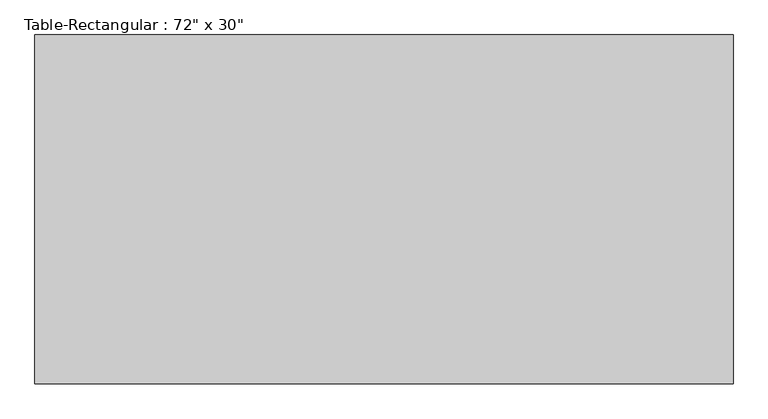
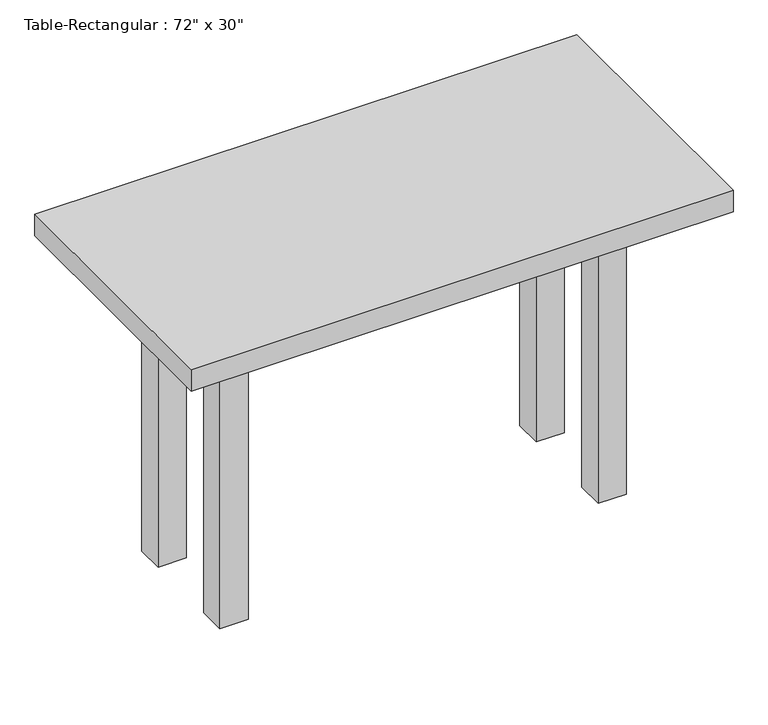
"""IFC4 building model written with IfcOpenShell, lengths in millimetres: furniture geometry."""

from ifc_helpers import new_model, si_unit, frame, origin, origin_with_axes, place, context, project, spatial, polyline, outline, extrude, source, transform, mapped, element, save


def furniture_51091a24(model_context):
    return source(origin(), model_context, "Body", "SweptSolid", [
        extrude(outline(polyline([(393.7, 114.3), (393.7, 88.9), (-393.7, 88.9), (-393.7, 114.3), (393.7, 114.3)])), frame((0.0, 0.0, 609.6), z_axis=(0.0, 0.0, 1.0), x_axis=(1.0, 0.0, 0.0)), (0.0, 0.0, 1.0), 101.6),
        extrude(outline(polyline([(393.7, -114.3), (-393.7, -114.3), (-393.7, -88.9), (393.7, -88.9), (393.7, -114.3)])), frame((0.0, 0.0, 609.6), z_axis=(0.0, 0.0, 1.0), x_axis=(1.0, 0.0, 0.0)), (0.0, 0.0, 1.0), 101.6),
        extrude(outline(polyline([(-406.4, -88.9), (-431.8, -88.9), (-431.8, 88.9), (-406.4, 88.9), (-406.4, -88.9)])), frame((0.0, 0.0, 609.6), z_axis=(0.0, 0.0, 1.0), x_axis=(1.0, 0.0, 0.0)), (0.0, 0.0, 1.0), 101.6),
        extrude(outline(polyline([(406.4, -88.9), (406.4, 88.9), (431.8, 88.9), (431.8, -88.9), (406.4, -88.9)])), frame((0.0, 0.0, 609.6), z_axis=(0.0, 0.0, 1.0), x_axis=(1.0, 0.0, 0.0)), (0.0, 0.0, 1.0), 101.6),
        extrude(outline(polyline([(609.6, 304.8), (609.6, -304.8), (-609.6, -304.8), (-609.6, 304.8), (609.6, 304.8)])), frame((0.0, 0.0, 711.2), z_axis=(0.0, 0.0, 1.0), x_axis=(1.0, 0.0, 0.0)), (0.0, 0.0, 1.0), 50.8),
        extrude(outline(polyline([(-393.7, 152.4), (-393.7, 88.9), (-457.2, 88.9), (-457.2, 152.4), (-393.7, 152.4)])), origin_with_axes(), (0.0, 0.0, 1.0), 711.2),
        extrude(outline(polyline([(393.7, 152.4), (457.2, 152.4), (457.2, 88.9), (393.7, 88.9), (393.7, 152.4)])), origin_with_axes(), (0.0, 0.0, 1.0), 711.2),
        extrude(outline(polyline([(-393.7, -152.4), (-457.2, -152.4), (-457.2, -88.9), (-393.7, -88.9), (-393.7, -152.4)])), origin_with_axes(), (0.0, 0.0, 1.0), 711.2),
        extrude(outline(polyline([(393.7, -152.4), (393.7, -88.9), (457.2, -88.9), (457.2, -152.4), (393.7, -152.4)])), origin_with_axes(), (0.0, 0.0, 1.0), 711.2),
    ])


if __name__ == "__main__":
    model = new_model("IFC4")
    model_context = context("Model", 3, world=origin())
    ifc_project = project(units=[si_unit("LENGTHUNIT", "METRE", prefix="MILLI")], contexts=[model_context])
    site = spatial("IfcSite", under=ifc_project)
    building = spatial("IfcBuilding", under=site)
    placement = place(None, origin())
    furniture_shape = furniture_51091a24(model_context)
    element("IfcFurniture", 1, ObjectType="Table-Rectangular : 72\" x 30\"", at=placement, inside=building, context=model_context, shape_type="MappedRepresentation", body=[
        mapped(furniture_shape, transform((0.0, 0.0, 0.0), x_axis=(1.0, 0.0, 0.0), y_axis=(0.0, 1.0, 0.0), z_axis=(0.0, 0.0, 1.0))),
    ])
    save(model, "model.ifc")

# Revit data of these elements
# Type "Table-Rectangular : 72\" x 30\""
#   Assembly Code = "E2020200"
#   Height = 2' - 6"
#   Length = 4' - 0"
#   Width = 2' - 0"
#   Base Material = Birch
#   Top Material = Birch
#   Default Elevation = 0
# Element 1 (IfcFurniture, "Table-Rectangular : 72\" x 30\"")
#   Materials on its faces: "Birch"
# Materials
#   "Birch": class "Wood", colour RGB 224 178 126, transparency 0, Description = "Betula Alleghaniensis", Cost = 0
